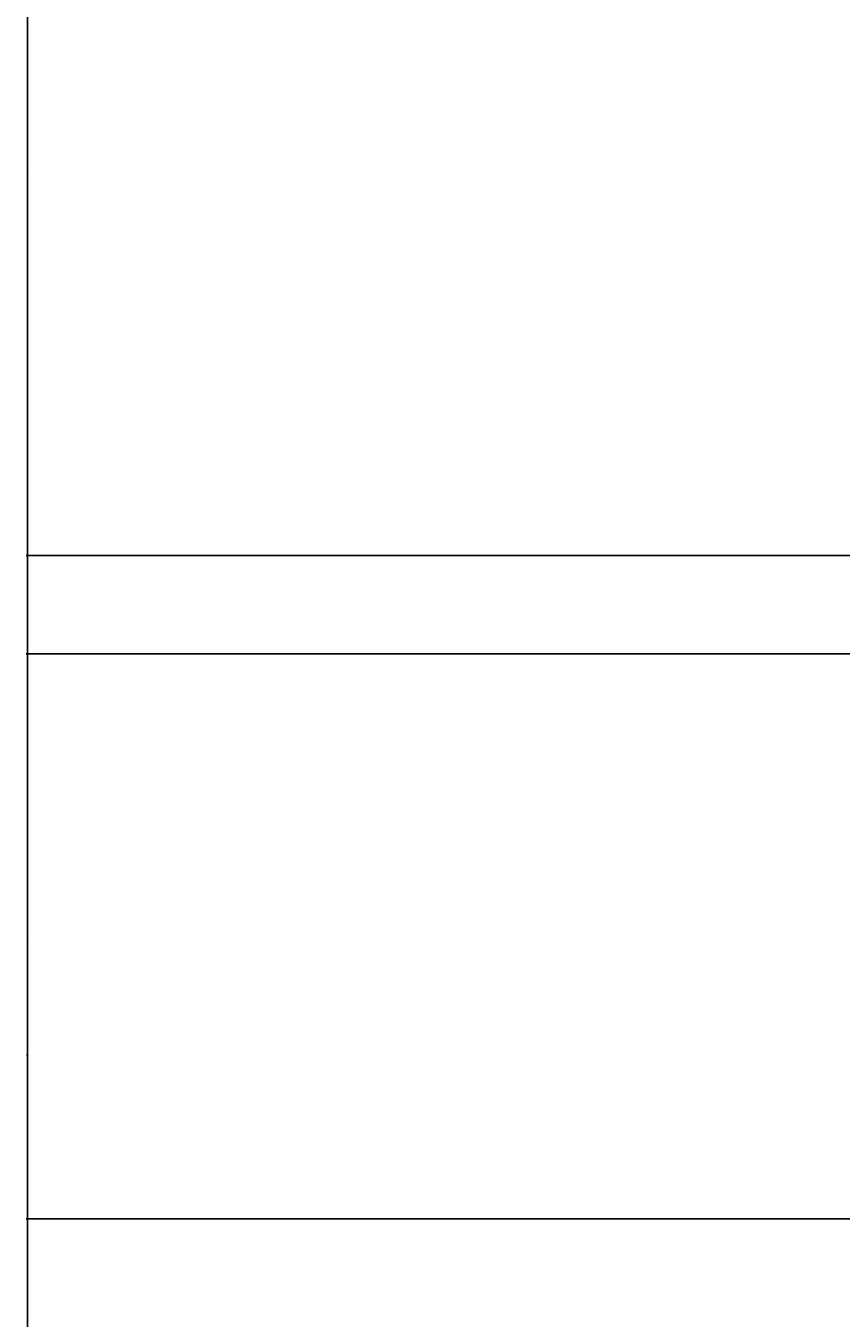
# Model space of a CAD drawing. Units: inches. Extents: x 5716 to 6907, y 12769 to 13594.
# Tile 3 of 17: x 5716 to 5815, y 13109 to 13266. Entities that reach past the tile are written whole.
import ezdxf

# ---------------------------------------------------------------- set-up
doc = ezdxf.new("R2010")
doc.units = ezdxf.units.IN
doc.layers.add('A-ANNO-DIMS', color=2, linetype='Continuous', lineweight=18)
doc.styles.get("Standard").update_dxf_attribs({"font": 'arial.ttf'})
doc.dimstyles.get("Standard").update_dxf_attribs({"dimtxt": 0.18, "dimasz": 0.18, "dimexe": 0.18, "dimexo": 0.0625, "dimgap": 0.09, "dimtad": 0, "dimtih": 1, "dimtoh": 1, "dimdec": 4, "dimzin": 0, "dimdsep": 46, "dimtxsty": 'Standard', "dimcen": 0.09, "dimadec": 0, "dimazin": 0, "dimtfac": 1, "dimtdec": 4, "dimtofl": 0, "dimtmove": 0, "dimatfit": 3, "dimfxl": 1, "dimtolj": 1, "dimtzin": 0, "dimarcsym": 0})

# ---------------------------------------------------------------- blocks, each defined once
blk = doc.blocks.new('*D50')
at = {"layer": 'A-ANNO-DIMS', "color": 0, "lineweight": -2, "transparency": 16777216}
for p, q in [((5818.96, 13440.15), (5716.04, 13440.15)), ((5716.22, 13439.97), (5716.22, 13140.83)), ((5716.22, 12841.33), (5716.22, 13140.47)), ((5818.96, 12841.15), (5716.04, 12841.15))]:
    blk.add_line(p, q, dxfattribs=at)
at = {"layer": 'A-ANNO-DIMS', "color": 0, "transparency": 16777216}
for points in [[(5716.19, 13439.97), (5716.25, 13439.97), (5716.22, 13440.15)], [(5716.19, 12841.33), (5716.25, 12841.33), (5716.22, 12841.15)]]:
    blk.add_solid(points, dxfattribs=at)
at = {"layer": 'Defpoints', "color": 0, "transparency": 16777216}
for p in [(5716.22, 13440.15), (5819.02, 13440.15), (5819.02, 12841.15)]:
    blk.add_point(p, dxfattribs=at)
at = {"layer": 'A-ANNO-DIMS', "color": 0, "transparency": 16777216, "insert": (5716.22, 13140.65), "char_height": 0.18, "attachment_point": 5}
blk.add_mtext('\\A1;599', dxfattribs=at)
blk = doc.blocks.new('*D52')
at = {"layer": 'A-ANNO-DIMS', "color": 0, "lineweight": -2, "transparency": 16777216}
for p, q in [((6267.34, 13440.15), (5716.04, 13440.15)), ((5716.22, 13439.97), (5716.22, 13140.83)), ((5716.22, 12841.33), (5716.22, 13140.47)), ((6267.34, 12841.15), (5716.04, 12841.15))]:
    blk.add_line(p, q, dxfattribs=at)
at = {"layer": 'A-ANNO-DIMS', "color": 0, "transparency": 16777216}
for points in [[(5716.19, 13439.97), (5716.25, 13439.97), (5716.22, 13440.15)], [(5716.19, 12841.33), (5716.25, 12841.33), (5716.22, 12841.15)]]:
    blk.add_solid(points, dxfattribs=at)
at = {"layer": 'Defpoints', "color": 0, "transparency": 16777216}
for p in [(6267.41, 13440.15), (5716.22, 12841.15), (6267.41, 12841.15)]:
    blk.add_point(p, dxfattribs=at)
at = {"layer": 'A-ANNO-DIMS', "color": 0, "transparency": 16777216, "insert": (5716.22, 13140.65), "char_height": 0.18, "attachment_point": 5}
blk.add_mtext('\\A1;599', dxfattribs=at)
blk = doc.blocks.new('*D59')
at = {"layer": 'A-ANNO-DIMS', "color": 0, "lineweight": -2, "transparency": 16777216}
for p, q in [((6736.67, 13294.65), (5716.04, 13294.65)), ((5716.22, 13294.47), (5716.22, 13248.33)), ((5716.22, 13201.83), (5716.22, 13247.97)), ((6736.67, 13201.65), (5716.04, 13201.65))]:
    blk.add_line(p, q, dxfattribs=at)
at = {"layer": 'A-ANNO-DIMS', "color": 0, "transparency": 16777216}
for points in [[(5716.19, 13294.47), (5716.25, 13294.47), (5716.22, 13294.65)], [(5716.19, 13201.83), (5716.25, 13201.83), (5716.22, 13201.65)]]:
    blk.add_solid(points, dxfattribs=at)
at = {"layer": 'Defpoints', "color": 0, "transparency": 16777216}
for p in [(6736.73, 13294.65), (5716.22, 13201.65), (6736.73, 13201.65)]:
    blk.add_point(p, dxfattribs=at)
at = {"layer": 'A-ANNO-DIMS', "color": 0, "transparency": 16777216, "insert": (5716.22, 13248.15), "char_height": 0.18, "attachment_point": 5}
blk.add_mtext('\\A1;93', dxfattribs=at)
blk = doc.blocks.new('*D60')
at = {"layer": 'A-ANNO-DIMS', "color": 0, "lineweight": -2, "transparency": 16777216}
for p, q in [((6736.67, 13201.65), (5716.04, 13201.65)), ((5716.22, 13201.47), (5716.22, 13195.83)), ((5716.22, 13189.83), (5716.22, 13195.47)), ((6827.78, 13189.65), (5716.04, 13189.65))]:
    blk.add_line(p, q, dxfattribs=at)
at = {"layer": 'A-ANNO-DIMS', "color": 0, "transparency": 16777216}
for points in [[(5716.19, 13201.47), (5716.25, 13201.47), (5716.22, 13201.65)], [(5716.19, 13189.83), (5716.25, 13189.83), (5716.22, 13189.65)]]:
    blk.add_solid(points, dxfattribs=at)
at = {"layer": 'Defpoints', "color": 0, "transparency": 16777216}
for p in [(6736.73, 13201.65), (5716.22, 13189.65), (6827.84, 13189.65)]:
    blk.add_point(p, dxfattribs=at)
at = {"layer": 'A-ANNO-DIMS', "color": 0, "transparency": 16777216, "insert": (5716.22, 13195.65), "char_height": 0.18, "attachment_point": 5}
blk.add_mtext('\\A1;12', dxfattribs=at)
blk = doc.blocks.new('*D61')
at = {"layer": 'A-ANNO-DIMS', "color": 0, "lineweight": -2, "transparency": 16777216}
for p, q in [((6827.78, 13189.65), (5716.04, 13189.65)), ((5716.22, 13189.47), (5716.22, 13155.33)), ((5716.22, 13120.83), (5716.22, 13154.97)), ((6736.67, 13120.65), (5716.04, 13120.65))]:
    blk.add_line(p, q, dxfattribs=at)
at = {"layer": 'A-ANNO-DIMS', "color": 0, "transparency": 16777216}
for points in [[(5716.19, 13189.47), (5716.25, 13189.47), (5716.22, 13189.65)], [(5716.19, 13120.83), (5716.25, 13120.83), (5716.22, 13120.65)]]:
    blk.add_solid(points, dxfattribs=at)
at = {"layer": 'Defpoints', "color": 0, "transparency": 16777216}
for p in [(6827.84, 13189.65), (5716.22, 13120.65), (6736.73, 13120.65)]:
    blk.add_point(p, dxfattribs=at)
at = {"layer": 'A-ANNO-DIMS', "color": 0, "transparency": 16777216, "insert": (5716.22, 13155.15), "char_height": 0.18, "attachment_point": 5}
blk.add_mtext('\\A1;69', dxfattribs=at)
blk = doc.blocks.new('*D62')
at = {"layer": 'A-ANNO-DIMS', "color": 0, "lineweight": -2, "transparency": 16777216}
for p, q in [((6736.67, 13120.65), (5716.04, 13120.65)), ((5716.22, 13120.47), (5716.22, 13100.33)), ((5716.22, 13079.83), (5716.22, 13099.97)), ((6736.67, 13079.65), (5716.04, 13079.65))]:
    blk.add_line(p, q, dxfattribs=at)
at = {"layer": 'A-ANNO-DIMS', "color": 0, "transparency": 16777216}
for points in [[(5716.19, 13120.47), (5716.25, 13120.47), (5716.22, 13120.65)], [(5716.19, 13079.83), (5716.25, 13079.83), (5716.22, 13079.65)]]:
    blk.add_solid(points, dxfattribs=at)
at = {"layer": 'Defpoints', "color": 0, "transparency": 16777216}
for p in [(6736.73, 13120.65), (5716.22, 13079.65), (6736.73, 13079.65)]:
    blk.add_point(p, dxfattribs=at)
at = {"layer": 'A-ANNO-DIMS', "color": 0, "transparency": 16777216, "insert": (5716.22, 13100.15), "char_height": 0.18, "attachment_point": 5}
blk.add_mtext('\\A1;41', dxfattribs=at)

msp = doc.modelspace()

# ---------------------------------------------------------------- dimensions: what is measured, and where the dimension line sits
at = {"layer": 'A-ANNO-DIMS'}
for base, p1, p2, picture, middle in [((5716.22, 13440.15), (5819.02, 12841.15), (5819.02, 13440.15), '*D50', (5716.22, 13140.65)), ((5716.22, 12841.15), (6267.41, 13440.15), (6267.41, 12841.15), '*D52', (5716.22, 13140.65)), ((5716.22, 13201.65), (6736.73, 13294.65), (6736.73, 13201.65), '*D59', (5716.22, 13248.15)), ((5716.22, 13189.65), (6736.73, 13201.65), (6827.84, 13189.65), '*D60', (5716.22, 13195.65)), ((5716.22, 13120.65), (6827.84, 13189.65), (6736.73, 13120.65), '*D61', (5716.22, 13155.15)), ((5716.22, 13079.65), (6736.73, 13120.65), (6736.73, 13079.65), '*D62', (5716.22, 13100.15))]:
    dim = msp.add_linear_dim(base=base, p1=p1, p2=p2, angle=90, dimstyle='Standard', override={"dimdec": 0, "dimlfac": 1, "dimrnd": 0, "dimzin": 0, "dimdsep": 46, "dimlunit": 2}, dxfattribs=at)
    dim.commit()
    dim.dimension.update_dxf_attribs({"geometry": picture, "text_midpoint": middle})

doc.saveas('drawing.dxf')
